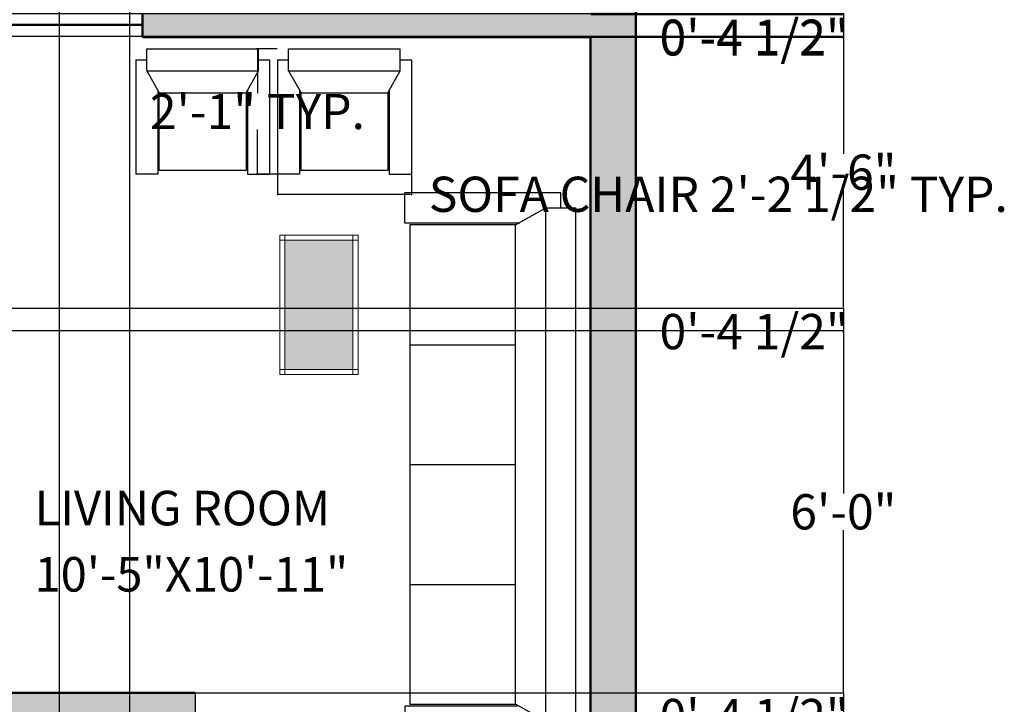
# Model space of a CAD drawing. Units: inches. Extents: x 48 to 822, y -191 to 651.
# Tile 12 of 13: x 626 to 822, y 297 to 433. Entities that reach past the tile are written whole.
import ezdxf

# ---------------------------------------------------------------- set-up
doc = ezdxf.new("R2010")
doc.units = ezdxf.units.IN
doc.header["$MEASUREMENT"] = 0
doc.layers.get('0').update_dxf_attribs({"color": 254})
for name, color, linetype, lineweight in [('A-ANNO-DIMS', 2, 'Continuous', 18), ('A-AREA-IDEN', 7, 'Continuous', 25), ('A-FLOR-STRS', 3, 'Continuous', 25), ('A-FURN', 8, 'Continuous', 18), ('A-WALL', 7, 'Continuous', 50), ('A-WALL-PATT', 8, 'Continuous', 13)]:
    doc.layers.add(name, color=color, linetype=linetype, lineweight=lineweight)
doc.layers.add('furniture', color=250, linetype='Continuous')
doc.styles.get("Standard").update_dxf_attribs({"font": 'arial.ttf'})
doc.dimstyles.get("Standard").update_dxf_attribs({"dimtxt": 7, "dimasz": 0.18, "dimexe": 0.18, "dimexo": 0.0625, "dimgap": 0.09, "dimtad": 0, "dimtih": 1, "dimtoh": 1, "dimzin": 0, "dimdsep": 46, "dimlunit": 3, "dimtxsty": 'Standard', "dimcen": 0.09, "dimadec": 0, "dimazin": 0, "dimtfac": 1, "dimtofl": 0, "dimtmove": 0, "dimatfit": 3, "dimfxl": 1, "dimtolj": 1, "dimtzin": 0, "dimarcsym": 0})

# ---------------------------------------------------------------- blocks, each defined once
blk = doc.blocks.new('FABRIC SOFA 1S')
at = {"layer": 'furniture'}
for p, q in [((3, 18.12), (34, 18.12)), ((3, 15.12), (3, 18.12)), ((34, 12.12), (34, 18.12)), ((0, -15.12), (0, 15.12)), ((6, 15.12), (0, 15.12)), ((6, -15.12), (6, 15.12)), ((12, 11.75), (6, 15.12)), ((11.33, 12.12), (34, 12.12)), ((6, -15.12), (12, -11.75)), ((11.33, -12.12), (34, -12.12)), ((34, -12.12), (34, -18.12)), ((6, -15.12), (0, -15.12)), ((3, -18.12), (3, -15.12)), ((3, -18.12), (34, -18.12))]:
    blk.add_line(p, q, dxfattribs=at)
blk.add_lwpolyline([(12, -11.75), (12, 11.75), (33, 11.75), (33, -11.75)], close=True, dxfattribs=at)
blk = doc.blocks.new('FABRIC SOFA 4S')
at = {"layer": 'furniture'}
for p, q in [((3, 54), (34, 54)), ((3, 51), (3, 54)), ((34, 48), (34, 54)), ((0, -51), (0, 51)), ((6, 51), (0, 51)), ((6, -51), (6, 51)), ((12, 47.63), (6, 51)), ((11.14, 48), (34, 48)), ((33, 23.81), (12, 23.81)), ((33, 0), (12, 0)), ((33, -23.81), (12, -23.81)), ((6, -51), (12, -47.63)), ((11.54, -48), (34, -48)), ((34, -48), (34, -54)), ((6, -51), (0, -51)), ((3, -54), (3, -51)), ((3, -54), (34, -54))]:
    blk.add_line(p, q, dxfattribs=at)
blk.add_lwpolyline([(12, -47.63), (12, 47.63), (33, 47.63), (33, -47.63)], close=True, dxfattribs=at)
blk = doc.blocks.new('COFFEE-TABLE')
for p, q in [((0, 27.69), (0, 0)), ((15.53, 27.69), (0, 27.69)), ((15.53, 0), (15.53, 27.69)), ((0, 0), (15.53, 0))]:
    blk.add_line(p, q)
blk = doc.blocks.new('*D46')
at = {"layer": 'A-ANNO-DIMS', "color": 0, "lineweight": -2, "transparency": 16777216}
for p, q in [((677.42, 402.71), (677.42, 398.61)), ((704.02, 402.71), (704.02, 398.61)), ((677.6, 398.79), (703.84, 398.79)), ((704.02, 398.79), (704.2, 398.79))]:
    blk.add_line(p, q, dxfattribs=at)
at = {"layer": 'A-ANNO-DIMS', "color": 0, "transparency": 16777216}
for points in [[(677.6, 398.82), (677.6, 398.76), (677.42, 398.79)], [(703.84, 398.82), (703.84, 398.76), (704.02, 398.79)]]:
    blk.add_solid(points, dxfattribs=at)
at = {"layer": 'Defpoints', "color": 0, "transparency": 16777216}
for p in [(677.42, 402.78), (704.02, 402.78), (704.02, 398.79)]:
    blk.add_point(p, dxfattribs=at)
at = {"layer": 'A-ANNO-DIMS', "color": 0, "transparency": 16777216, "insert": (765.01, 398.79), "char_height": 7, "attachment_point": 5}
blk.add_mtext('\\A1;SOFA CHAIR 2\'-2 1/2" TYP.', dxfattribs=at)
blk = doc.blocks.new('*D47')
at = {"layer": 'A-ANNO-DIMS', "color": 0, "lineweight": -2, "transparency": 16777216}
for p, q in [((677.36, 427.73), (673.25, 427.73)), ((673.43, 427.55), (673.43, 418.86)), ((673.43, 402.96), (673.43, 411.65)), ((677.36, 402.78), (673.25, 402.78))]:
    blk.add_line(p, q, dxfattribs=at)
at = {"layer": 'A-ANNO-DIMS', "color": 0, "transparency": 16777216}
for points in [[(673.4, 427.55), (673.46, 427.55), (673.43, 427.73)], [(673.4, 402.96), (673.46, 402.96), (673.43, 402.78)]]:
    blk.add_solid(points, dxfattribs=at)
at = {"layer": 'Defpoints', "color": 0, "transparency": 16777216}
for p in [(677.42, 427.73), (673.43, 402.78), (677.42, 402.78)]:
    blk.add_point(p, dxfattribs=at)
at = {"layer": 'A-ANNO-DIMS', "color": 0, "transparency": 16777216, "insert": (673.43, 415.25), "char_height": 7, "attachment_point": 5}
blk.add_mtext('\\A1;2\'-1" TYP.', dxfattribs=at)
blk = doc.blocks.new('*D106')
at = {"layer": 'A-ANNO-DIMS', "color": 0, "lineweight": -2, "transparency": 16777216}
for p, q in [((517.67, 434.69), (790.04, 434.69)), ((789.86, 434.51), (789.86, 430.37)), ((517.67, 430.19), (790.04, 430.19)), ((789.86, 430.01), (789.68, 430.01)), ((789.86, 430.19), (789.86, 430.01))]:
    blk.add_line(p, q, dxfattribs=at)
at = {"layer": 'A-ANNO-DIMS', "color": 0, "transparency": 16777216}
for points in [[(789.83, 434.51), (789.89, 434.51), (789.86, 434.69)], [(789.83, 430.37), (789.89, 430.37), (789.86, 430.19)]]:
    blk.add_solid(points, dxfattribs=at)
at = {"layer": 'Defpoints', "color": 0, "transparency": 16777216}
for p in [(517.61, 434.69), (517.61, 430.19), (789.86, 430.19)]:
    blk.add_point(p, dxfattribs=at)
at = {"layer": 'A-ANNO-DIMS', "color": 0, "transparency": 16777216, "insert": (772.13, 430.01), "char_height": 7, "attachment_point": 5}
blk.add_mtext('\\A1;0\'-4 1/2"', dxfattribs=at)
blk = doc.blocks.new('*D107')
at = {"layer": 'A-ANNO-DIMS', "color": 0, "lineweight": -2, "transparency": 16777216}
for p, q in [((517.67, 430.19), (790.04, 430.19)), ((789.86, 430.01), (789.86, 406.85)), ((789.86, 376.37), (789.86, 399.52)), ((517.67, 376.19), (790.04, 376.19))]:
    blk.add_line(p, q, dxfattribs=at)
at = {"layer": 'A-ANNO-DIMS', "color": 0, "transparency": 16777216}
for points in [[(789.83, 430.01), (789.89, 430.01), (789.86, 430.19)], [(789.83, 376.37), (789.89, 376.37), (789.86, 376.19)]]:
    blk.add_solid(points, dxfattribs=at)
at = {"layer": 'Defpoints', "color": 0, "transparency": 16777216}
for p in [(517.61, 430.19), (517.61, 376.19), (789.86, 376.19)]:
    blk.add_point(p, dxfattribs=at)
at = {"layer": 'A-ANNO-DIMS', "color": 0, "transparency": 16777216, "insert": (789.86, 403.19), "char_height": 7, "attachment_point": 5}
blk.add_mtext('\\A1;4\'-6"', dxfattribs=at)
blk = doc.blocks.new('*D108')
at = {"layer": 'A-ANNO-DIMS', "color": 0, "lineweight": -2, "transparency": 16777216}
for p, q in [((517.67, 376.19), (790.04, 376.19)), ((789.86, 376.01), (789.86, 371.87)), ((517.67, 371.69), (790.04, 371.69)), ((789.86, 371.51), (789.68, 371.51)), ((789.86, 371.69), (789.86, 371.51))]:
    blk.add_line(p, q, dxfattribs=at)
at = {"layer": 'A-ANNO-DIMS', "color": 0, "transparency": 16777216}
for points in [[(789.83, 376.01), (789.89, 376.01), (789.86, 376.19)], [(789.83, 371.87), (789.89, 371.87), (789.86, 371.69)]]:
    blk.add_solid(points, dxfattribs=at)
at = {"layer": 'Defpoints', "color": 0, "transparency": 16777216}
for p in [(517.61, 376.19), (517.61, 371.69), (789.86, 371.69)]:
    blk.add_point(p, dxfattribs=at)
at = {"layer": 'A-ANNO-DIMS', "color": 0, "transparency": 16777216, "insert": (772.13, 371.51), "char_height": 7, "attachment_point": 5}
blk.add_mtext('\\A1;0\'-4 1/2"', dxfattribs=at)
blk = doc.blocks.new('*D109')
at = {"layer": 'A-ANNO-DIMS', "color": 0, "lineweight": -2, "transparency": 16777216}
for p, q in [((517.67, 371.69), (790.04, 371.69)), ((789.86, 371.51), (789.86, 339.35)), ((789.86, 299.87), (789.86, 332.02)), ((517.67, 299.69), (790.04, 299.69))]:
    blk.add_line(p, q, dxfattribs=at)
at = {"layer": 'A-ANNO-DIMS', "color": 0, "transparency": 16777216}
for points in [[(789.83, 371.51), (789.89, 371.51), (789.86, 371.69)], [(789.83, 299.87), (789.89, 299.87), (789.86, 299.69)]]:
    blk.add_solid(points, dxfattribs=at)
at = {"layer": 'Defpoints', "color": 0, "transparency": 16777216}
for p in [(517.61, 371.69), (517.61, 299.69), (789.86, 299.69)]:
    blk.add_point(p, dxfattribs=at)
at = {"layer": 'A-ANNO-DIMS', "color": 0, "transparency": 16777216, "insert": (789.86, 335.69), "char_height": 7, "attachment_point": 5}
blk.add_mtext('\\A1;6\'-0"', dxfattribs=at)
blk = doc.blocks.new('*D110')
at = {"layer": 'A-ANNO-DIMS', "color": 0, "lineweight": -2, "transparency": 16777216}
for p, q in [((517.67, 299.69), (790.04, 299.69)), ((789.86, 299.51), (789.86, 295.37)), ((517.67, 295.19), (790.04, 295.19)), ((789.86, 295.01), (789.68, 295.01)), ((789.86, 295.19), (789.86, 295.01))]:
    blk.add_line(p, q, dxfattribs=at)
at = {"layer": 'A-ANNO-DIMS', "color": 0, "transparency": 16777216}
for points in [[(789.83, 299.51), (789.89, 299.51), (789.86, 299.69)], [(789.83, 295.37), (789.89, 295.37), (789.86, 295.19)]]:
    blk.add_solid(points, dxfattribs=at)
at = {"layer": 'Defpoints', "color": 0, "transparency": 16777216}
for p in [(517.61, 299.69), (517.61, 295.19), (789.86, 295.19)]:
    blk.add_point(p, dxfattribs=at)
at = {"layer": 'A-ANNO-DIMS', "color": 0, "transparency": 16777216, "insert": (772.13, 295.01), "char_height": 7, "attachment_point": 5}
blk.add_mtext('\\A1;0\'-4 1/2"', dxfattribs=at)
blk = doc.blocks.new('*D121')
at = {"layer": 'A-ANNO-DIMS', "color": 0, "lineweight": -2, "transparency": 16777216}
for p, q in [((739.67, 434.54), (790.04, 434.54)), ((789.86, 434.36), (789.86, 430.22)), ((739.67, 430.04), (790.04, 430.04)), ((789.86, 429.86), (789.68, 429.86)), ((789.86, 430.04), (789.86, 429.86))]:
    blk.add_line(p, q, dxfattribs=at)
at = {"layer": 'A-ANNO-DIMS', "color": 0, "transparency": 16777216}
for points in [[(789.83, 434.36), (789.89, 434.36), (789.86, 434.54)], [(789.83, 430.22), (789.89, 430.22), (789.86, 430.04)]]:
    blk.add_solid(points, dxfattribs=at)
at = {"layer": 'Defpoints', "color": 0, "transparency": 16777216}
for p in [(739.61, 434.54), (739.61, 430.04), (789.86, 430.04)]:
    blk.add_point(p, dxfattribs=at)
at = {"layer": 'A-ANNO-DIMS', "color": 0, "transparency": 16777216, "insert": (772.13, 429.86), "char_height": 7, "attachment_point": 5}
blk.add_mtext('\\A1;0\'-4 1/2"', dxfattribs=at)
blk = doc.blocks.new('*D125')
at = {"layer": 'A-ANNO-DIMS', "color": 0, "lineweight": -2, "transparency": 16777216}
for p, q in [((634.1, 295.25), (634.1, 641.12)), ((634.28, 640.94), (647.91, 640.94)), ((648.09, 295.25), (648.09, 641.12)), ((648.09, 640.94), (648.27, 640.94))]:
    blk.add_line(p, q, dxfattribs=at)
at = {"layer": 'A-ANNO-DIMS', "color": 0, "transparency": 16777216}
for points in [[(634.28, 640.97), (634.28, 640.91), (634.1, 640.94)], [(647.91, 640.97), (647.91, 640.91), (648.09, 640.94)]]:
    blk.add_solid(points, dxfattribs=at)
at = {"layer": 'Defpoints', "color": 0, "transparency": 16777216}
for p in [(648.09, 640.94), (634.1, 295.19), (648.09, 295.19)]:
    blk.add_point(p, dxfattribs=at)
at = {"layer": 'A-ANNO-DIMS', "color": 0, "transparency": 16777216, "insert": (657.33, 640.94), "char_height": 7, "attachment_point": 5}
blk.add_mtext('\\A1;1\'-2"', dxfattribs=at)
blk = doc.blocks.new('*D126')
at = {"layer": 'A-ANNO-DIMS', "color": 0, "lineweight": -2, "transparency": 16777216}
for p, q in [((553.61, 295.25), (553.61, 641.12)), ((553.79, 640.94), (580.61, 640.94)), ((647.91, 640.94), (621.09, 640.94)), ((648.09, 295.25), (648.09, 641.12))]:
    blk.add_line(p, q, dxfattribs=at)
at = {"layer": 'A-ANNO-DIMS', "color": 0, "transparency": 16777216}
for points in [[(553.79, 640.97), (553.79, 640.91), (553.61, 640.94)], [(647.91, 640.97), (647.91, 640.91), (648.09, 640.94)]]:
    blk.add_solid(points, dxfattribs=at)
at = {"layer": 'Defpoints', "color": 0, "transparency": 16777216}
for p in [(648.09, 640.94), (553.61, 295.19), (648.09, 295.19)]:
    blk.add_point(p, dxfattribs=at)
at = {"layer": 'A-ANNO-DIMS', "color": 0, "transparency": 16777216, "insert": (600.85, 640.94), "char_height": 7, "attachment_point": 5}
blk.add_mtext('\\A1;7\'-10 1/2"', dxfattribs=at)

msp = doc.modelspace()

# ---------------------------------------------------------------- hatches: boundary and pattern name
at = {"layer": 'A-FURN'}
h = msp.add_hatch(color=256, dxfattribs=at)
h.dxf.hatch_style = 1
h.paths.add_polyline_path([(692.415, 389.686), (678.89, 389.686), (678.89, 363.994), (692.415, 363.994)])
at = {"layer": 'A-WALL-PATT'}
h = msp.add_hatch(color=256, dxfattribs=at)
h.dxf.hatch_style = 1
h.paths.add_polyline_path([(614.11, 432.437), (609.61, 432.437), (609.61, 376.187), (535.284, 376.187), (535.284, 371.687), (547.61, 371.687), (547.61, 359.12), (552.11, 359.12), (552.11, 371.687), (609.61, 371.687), (609.61, 335.687), (614.11, 335.687)], flags=17)
h.paths.add_polyline_path([(614.11, 434.687), (609.61, 434.687), (609.61, 432.437), (614.11, 432.437)], flags=17)
h.paths.add_polyline_path([(573.934, 434.687), (517.61, 434.687), (517.61, 590.687), (650.61, 590.687), (650.61, 585.522), (655.11, 585.522), (655.11, 590.687), (739.61, 590.687), (739.61, 548.687), (655.11, 548.687), (655.11, 550.72), (650.61, 550.72), (650.61, 458.608), (655.11, 458.608), (655.11, 544.187), (739.61, 544.187), (739.61, 434.541), (650.61, 434.541), (650.61, 430.041), (739.61, 430.041), (739.61, -16.844), (729.973, -16.844), (729.973, -21.344), (748.61, -21.344), (748.61, 599.687), (508.61, 599.687), (508.61, -120.313), (543.114, -120.313), (543.114, -111.313), (517.61, -111.313), (517.61, 38.687), (607.29, 38.687), (607.29, 43.187), (517.61, 43.187), (517.61, 97.187), (654.61, 97.187), (654.61, 30.562), (659.11, 30.562), (659.11, 101.895), (654.61, 101.895), (654.61, 101.687), (517.61, 101.687), (517.61, 221.687), (654.61, 221.687), (654.61, 218.066), (659.11, 218.066), (659.11, 226.187), (517.61, 226.187), (517.61, 295.187), (614.11, 295.187), (648.087, 295.187), (661.07, 295.187), (661.07, 299.687), (614.11, 299.687), (552.11, 299.687), (552.11, 341.37), (547.61, 341.37), (547.61, 299.687), (517.61, 299.687), (517.61, 371.687), (517.534, 371.687), (517.534, 376.187), (517.61, 430.187), (573.934, 430.187)])
h.paths.add_polyline_path([(659.11, -87.328), (654.61, -87.328), (654.61, -111.313), (598.94, -111.313), (598.94, -120.313), (659.11, -120.313)], flags=0)
h.paths.add_polyline_path([(671.266, -16.844), (659.11, -16.844), (659.11, -12.05), (654.61, -12.05), (654.61, -31.502), (659.11, -31.502), (659.11, -21.344), (671.266, -21.344)], flags=17)
h.paths.add_polyline_path([(606.11, 97.187), (601.61, 97.187), (601.61, 75.902), (606.11, 75.902)], flags=17)
h.paths.add_polyline_path([(659.11, 169.875), (654.61, 169.875), (654.61, 157.721), (659.11, 157.721)], flags=17)

# ---------------------------------------------------------------- linework, layer by layer
at = {"layer": 'A-FLOR-STRS'}
msp.add_line((661.07, 299.687), (661.07, 295.187), dxfattribs=at)
at = {"layer": 'A-FURN'}
for p, q in [((693.415, 389.686), (677.89, 389.686)), ((678.89, 390.686), (678.89, 362.994)), ((692.415, 362.994), (692.415, 390.686)), ((677.89, 363.994), (693.415, 363.994))]:
    msp.add_line(p, q, dxfattribs=at)
at = {"layer": 'A-WALL'}
for p, q in [((748.61, 599.687), (748.61, -120.313)), ((650.61, 434.541), (650.61, 430.041)), ((614.11, 432.437), (650.61, 432.437)), ((650.61, 430.041), (739.61, 430.041)), ((739.61, 430.041), (739.61, -16.844)), ((614.11, 299.687), (661.07, 299.687))]:
    msp.add_line(p, q, dxfattribs=at)

# ---------------------------------------------------------------- block references
at = {"layer": 'A-FURN', "xscale": 0.7339463821036302, "yscale": 0.7339463821036302, "zscale": 0.7339463821036302, "rotation": 270}
for p in [(662.558, 427.73), (690.721, 427.73)]:
    msp.add_blockref('FABRIC SOFA 1S', p, dxfattribs=at)
at = {"layer": 'A-FURN', "xscale": -1}
msp.add_blockref('FABRIC SOFA 4S', (736.72, 345.068), dxfattribs=at)
at = {"layer": 'A-FURN'}
msp.add_blockref('COFFEE-TABLE', (677.89, 362.993), dxfattribs=at)

# ---------------------------------------------------------------- texts
at = {"layer": 'A-AREA-IDEN'}
for s, p in [('LIVING ROOM', (629.141, 332.998)), ('10\'-5"X10\'-11"', (629.141, 319.839))]:
    msp.add_text(s, height=6.86603, dxfattribs=at).set_placement(p)

# ---------------------------------------------------------------- dimensions: what is measured, and where the dimension line sits
at = {"layer": 'A-ANNO-DIMS'}
for p1, picture, middle in [((553.61, 295.187), '*D126', (600.849, 640.937)), ((634.101, 295.187), '*D125', (657.331, 640.937))]:
    dim = msp.add_linear_dim(base=(648.087, 640.937), p1=p1, p2=(648.087, 295.187), dimstyle='Standard', override={"dimdec": 1, "dimlfac": 1, "dimrnd": 0, "dimzin": 1, "dimdsep": 46, "dimlunit": 4, "dimfrac": 2}, dxfattribs=at)
    dim.commit()
    dim.dimension.update_dxf_attribs({"geometry": picture, "text_midpoint": middle})
for base, p1, p2, picture, middle in [((789.86, 430.187), (517.61, 434.687), (517.61, 430.187), '*D106', (772.131, 430.007)), ((789.86, 430.041), (739.61, 434.541), (739.61, 430.041), '*D121', (772.131, 429.861)), ((789.86, 376.187), (517.61, 430.187), (517.61, 376.187), '*D107', (789.86, 403.187)), ((789.86, 371.687), (517.61, 376.187), (517.61, 371.687), '*D108', (772.131, 371.507)), ((789.86, 299.687), (517.61, 371.687), (517.61, 299.687), '*D109', (789.86, 335.687)), ((789.86, 295.187), (517.61, 299.687), (517.61, 295.187), '*D110', (772.131, 295.007))]:
    dim = msp.add_linear_dim(base=base, p1=p1, p2=p2, angle=90, dimstyle='Standard', override={"dimdec": 1, "dimlfac": 1, "dimrnd": 0, "dimzin": 1, "dimdsep": 46, "dimlunit": 4, "dimfrac": 2}, dxfattribs=at)
    dim.commit()
    dim.dimension.update_dxf_attribs({"geometry": picture, "text_midpoint": middle})
dim = msp.add_linear_dim(base=(673.427, 402.776), p1=(677.418, 427.73), p2=(677.418, 402.776), angle=270, text='<> TYP.', dimstyle='Standard', override={"dimdec": 1, "dimlfac": 1, "dimrnd": 0, "dimzin": 1, "dimdsep": 46, "dimlunit": 4, "dimfrac": 2}, dxfattribs=at)
dim.commit()
dim.dimension.update_dxf_attribs({"geometry": '*D47', "text_midpoint": (673.427, 415.253)})
dim = msp.add_linear_dim(base=(704.023, 398.785), p1=(677.418, 402.776), p2=(704.023, 402.776), text='SOFA CHAIR <> TYP.', dimstyle='Standard', override={"dimdec": 1, "dimlfac": 1, "dimrnd": 0, "dimzin": 1, "dimdsep": 46, "dimlunit": 4, "dimfrac": 2}, dxfattribs=at)
dim.commit()
dim.dimension.update_dxf_attribs({"geometry": '*D46', "text_midpoint": (765.009, 398.785)})

doc.saveas('drawing.dxf')
